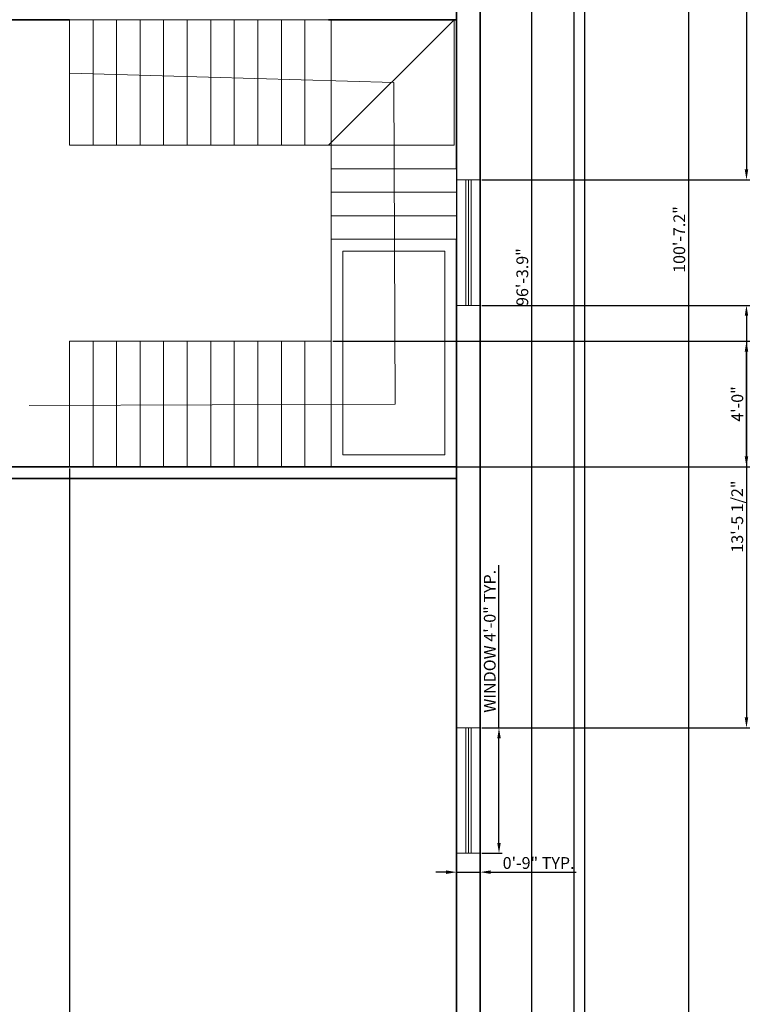
# Model space of a CAD drawing. Units: inches. Extents: x 1239 to 2276906, y 2273 to 321338.
# Tile 14 of 23: x 1754 to 2036, y 2650 to 3026. Entities that reach past the tile are written whole.
import ezdxf

# ---------------------------------------------------------------- set-up
doc = ezdxf.new("R2010")
doc.units = ezdxf.units.IN
for name, color, linetype, lineweight in [('A-ANNO-DIMS', 2, 'Continuous', 18), ('C-PROP', 7, 'Continuous', 25), ('STAIRCASE', 3, 'Continuous', 18), ('wall', 7, 'Continuous', 35), ('WINDOW', 50, 'Continuous', 18)]:
    doc.layers.add(name, color=color, linetype=linetype, lineweight=lineweight)
doc.styles.get("Standard").update_dxf_attribs({"font": 'arial.ttf'})
doc.dimstyles.new('ISO-25', dxfattribs={"dimtxt": 4.5, "dimasz": 4, "dimexe": 1.25, "dimexo": 0.625, "dimtad": 1, "dimdec": 1, "dimlunit": 3, "dimtxsty": 'Standard', "dimcen": 2.5, "dimadec": 0, "dimazin": 0, "dimtfac": 1, "dimtdec": 1, "dimtmove": 0, "dimatfit": 3, "dimfxl": 1, "dimarcsym": 0})

# ---------------------------------------------------------------- blocks, each defined once
blk = doc.blocks.new('*D38')
at = {"layer": 'A-ANNO-DIMS', "color": 0, "lineweight": -2, "transparency": 16777216}
for p, q in [((1971.01, 3545.9), (2011.25, 3545.9)), ((2010, 3541.9), (2010, 2342.75)), ((1971.01, 2338.75), (2011.25, 2338.75))]:
    blk.add_line(p, q, dxfattribs=at)
at = {"layer": 'A-ANNO-DIMS', "color": 0, "transparency": 16777216}
for points in [[(2009.33, 3541.9), (2010.67, 3541.9), (2010, 3545.9)], [(2009.33, 2342.75), (2010.67, 2342.75), (2010, 2338.75)]]:
    blk.add_solid(points, dxfattribs=at)
at = {"layer": 'Defpoints', "color": 0, "transparency": 16777216}
for p in [(1970.38, 3545.9), (1970.38, 2338.75), (2010, 2338.75)]:
    blk.add_point(p, dxfattribs=at)
at = {"layer": 'A-ANNO-DIMS', "color": 0, "transparency": 16777216, "insert": (2007.08, 2942.32), "char_height": 4.5, "attachment_point": 5, "rotation": 90}
blk.add_mtext('100\'-7.2"', dxfattribs=at)
blk = doc.blocks.new('*D40')
at = {"layer": 'A-ANNO-DIMS', "color": 0, "lineweight": -2, "transparency": 16777216}
for p, q in [((1931.01, 3505.9), (1951.25, 3505.9)), ((1950, 3501.9), (1950, 2354)), ((1931.01, 2350), (1951.25, 2350))]:
    blk.add_line(p, q, dxfattribs=at)
at = {"layer": 'A-ANNO-DIMS', "color": 0, "transparency": 16777216}
for points in [[(1949.33, 3501.9), (1950.67, 3501.9), (1950, 3505.9)], [(1949.33, 2354), (1950.67, 2354), (1950, 2350)]]:
    blk.add_solid(points, dxfattribs=at)
at = {"layer": 'Defpoints', "color": 0, "transparency": 16777216}
for p in [(1930.38, 3505.9), (1930.38, 2350), (1950, 2350)]:
    blk.add_point(p, dxfattribs=at)
at = {"layer": 'A-ANNO-DIMS', "color": 0, "transparency": 16777216, "insert": (1947.08, 2927.95), "char_height": 4.5, "attachment_point": 5, "rotation": 90}
blk.add_mtext('96\'-3.9"', dxfattribs=at)
blk = doc.blocks.new('WIN-48')
for p, q in [((0, 48), (9, 48)), ((0, 0), (0, 48)), ((3.5, 0), (3.5, 48)), ((4.5, 0), (4.5, 48)), ((5.5, 0), (5.5, 48)), ((9, 0), (9, 48)), ((0, 0), (9, 0))]:
    blk.add_line(p, q)
blk = doc.blocks.new('*D46')
at = {"layer": 'A-ANNO-DIMS', "color": 0, "lineweight": -2, "transparency": 16777216}
for p, q in [((1937.58, 2755.54), (1937.58, 2817.73)), ((1931.01, 2755.54), (1938.83, 2755.54)), ((1937.58, 2711.54), (1937.58, 2751.54)), ((1931.01, 2707.54), (1938.83, 2707.54))]:
    blk.add_line(p, q, dxfattribs=at)
at = {"layer": 'A-ANNO-DIMS', "color": 0, "transparency": 16777216}
for points in [[(1936.92, 2751.54), (1938.25, 2751.54), (1937.58, 2755.54)], [(1936.92, 2711.54), (1938.25, 2711.54), (1937.58, 2707.54)]]:
    blk.add_solid(points, dxfattribs=at)
at = {"layer": 'Defpoints', "color": 0, "transparency": 16777216}
for p in [(1930.38, 2755.54), (1937.58, 2755.54), (1930.38, 2707.54)]:
    blk.add_point(p, dxfattribs=at)
at = {"layer": 'A-ANNO-DIMS', "color": 0, "transparency": 16777216, "insert": (1934.63, 2788.64), "char_height": 4.5, "attachment_point": 5, "rotation": 90}
blk.add_mtext('WINDOW 4\'-0" TYP.', dxfattribs=at)
blk = doc.blocks.new('*D47')
at = {"layer": 'A-ANNO-DIMS', "color": 0, "lineweight": -2, "transparency": 16777216}
for p, q in [((1921.38, 2706.91), (1921.38, 2699.09)), ((1930.38, 2706.91), (1930.38, 2699.09)), ((1917.38, 2700.34), (1913.38, 2700.34)), ((1921.38, 2700.34), (1930.38, 2700.34)), ((1934.38, 2700.34), (1967.06, 2700.34))]:
    blk.add_line(p, q, dxfattribs=at)
at = {"layer": 'A-ANNO-DIMS', "color": 0, "transparency": 16777216}
for points in [[(1917.38, 2701.01), (1917.38, 2699.67), (1921.38, 2700.34)], [(1934.38, 2701.01), (1934.38, 2699.67), (1930.38, 2700.34)]]:
    blk.add_solid(points, dxfattribs=at)
at = {"layer": 'Defpoints', "color": 0, "transparency": 16777216}
for p in [(1921.38, 2707.54), (1930.38, 2707.54), (1930.38, 2700.34)]:
    blk.add_point(p, dxfattribs=at)
at = {"layer": 'A-ANNO-DIMS', "color": 0, "transparency": 16777216, "insert": (1952.72, 2703.26), "char_height": 4.5, "attachment_point": 5}
blk.add_mtext('0\'-9" TYP.', dxfattribs=at)
blk = doc.blocks.new('*D87')
at = {"layer": 'A-ANNO-DIMS', "color": 0, "lineweight": -2, "transparency": 16777216}
for p, q in [((1666.38, 3250.77), (1666.38, 2275.7)), ((1921.38, 3250.77), (1921.38, 2275.7)), ((1670.38, 2276.95), (1917.38, 2276.95))]:
    blk.add_line(p, q, dxfattribs=at)
at = {"layer": 'A-ANNO-DIMS', "color": 0, "transparency": 16777216}
for points in [[(1670.38, 2277.61), (1670.38, 2276.28), (1666.38, 2276.95)], [(1917.38, 2277.61), (1917.38, 2276.28), (1921.38, 2276.95)]]:
    blk.add_solid(points, dxfattribs=at)
at = {"layer": 'Defpoints', "color": 0, "transparency": 16777216}
for p in [(1666.38, 3251.4), (1921.38, 3251.4), (1921.38, 2276.95)]:
    blk.add_point(p, dxfattribs=at)
at = {"layer": 'A-ANNO-DIMS', "color": 0, "transparency": 16777216, "insert": (1793.88, 2279.87), "char_height": 4.5, "attachment_point": 5}
blk.add_mtext('21\'-3"', dxfattribs=at)
blk = doc.blocks.new('*D98')
at = {"layer": 'A-ANNO-DIMS', "color": 0, "lineweight": -2, "transparency": 16777216}
for p, q in [((1772.76, 3026.4), (1247.33, 3026.4)), ((1248.58, 2859.4), (1248.58, 3022.4)), ((1772.76, 2855.4), (1247.33, 2855.4))]:
    blk.add_line(p, q, dxfattribs=at)
at = {"layer": 'A-ANNO-DIMS', "color": 0, "transparency": 16777216}
for points in [[(1247.92, 3022.4), (1249.25, 3022.4), (1248.58, 3026.4)], [(1247.92, 2859.4), (1249.25, 2859.4), (1248.58, 2855.4)]]:
    blk.add_solid(points, dxfattribs=at)
at = {"layer": 'Defpoints', "color": 0, "transparency": 16777216}
for p in [(1248.58, 3026.4), (1773.38, 3026.4), (1773.38, 2855.4)]:
    blk.add_point(p, dxfattribs=at)
at = {"layer": 'A-ANNO-DIMS', "color": 0, "transparency": 16777216, "insert": (1245.66, 2940.9), "char_height": 4.5, "attachment_point": 5, "rotation": 90}
blk.add_mtext('14\'-3"', dxfattribs=at)
blk = doc.blocks.new('*D99')
at = {"layer": 'A-ANNO-DIMS', "color": 0, "lineweight": -2, "transparency": 16777216}
for p, q in [((1773.38, 2854.77), (1773.38, 2275.7)), ((1921.38, 2854.77), (1921.38, 2275.7)), ((1777.38, 2276.95), (1917.38, 2276.95))]:
    blk.add_line(p, q, dxfattribs=at)
at = {"layer": 'A-ANNO-DIMS', "color": 0, "transparency": 16777216}
for points in [[(1777.38, 2277.61), (1777.38, 2276.28), (1773.38, 2276.95)], [(1917.38, 2277.61), (1917.38, 2276.28), (1921.38, 2276.95)]]:
    blk.add_solid(points, dxfattribs=at)
at = {"layer": 'Defpoints', "color": 0, "transparency": 16777216}
for p in [(1773.38, 2855.4), (1921.38, 2855.4), (1921.38, 2276.95)]:
    blk.add_point(p, dxfattribs=at)
at = {"layer": 'A-ANNO-DIMS', "color": 0, "transparency": 16777216, "insert": (1847.38, 2279.83), "char_height": 4.5, "attachment_point": 5}
blk.add_mtext('12\'-4"', dxfattribs=at)
blk = doc.blocks.new('*D109')
at = {"layer": 'A-ANNO-DIMS', "color": 0, "lineweight": -2, "transparency": 16777216}
for p, q in [((1931.01, 3298.46), (2033.43, 3298.46)), ((2032.18, 3294.46), (2032.18, 2969.13)), ((1931.01, 2965.13), (2033.43, 2965.13))]:
    blk.add_line(p, q, dxfattribs=at)
at = {"layer": 'A-ANNO-DIMS', "color": 0, "transparency": 16777216}
for points in [[(2031.52, 3294.46), (2032.85, 3294.46), (2032.18, 3298.46)], [(2031.52, 2969.13), (2032.85, 2969.13), (2032.18, 2965.13)]]:
    blk.add_solid(points, dxfattribs=at)
at = {"layer": 'Defpoints', "color": 0, "transparency": 16777216}
for p in [(1930.38, 3298.46), (1930.38, 2965.13), (2032.18, 2965.13)]:
    blk.add_point(p, dxfattribs=at)
at = {"layer": 'A-ANNO-DIMS', "color": 0, "transparency": 16777216, "insert": (2029.23, 3131.8), "char_height": 4.5, "attachment_point": 5, "rotation": 90}
blk.add_mtext('27\'-9 1/2"', dxfattribs=at)
blk = doc.blocks.new('*D110')
at = {"layer": 'A-ANNO-DIMS', "color": 0, "lineweight": -2, "transparency": 16777216}
for p, q in [((1931.01, 2917.13), (2033.43, 2917.13)), ((2032.18, 2913.13), (2032.18, 2759.54)), ((1931.01, 2755.54), (2033.43, 2755.54))]:
    blk.add_line(p, q, dxfattribs=at)
at = {"layer": 'A-ANNO-DIMS', "color": 0, "transparency": 16777216}
for points in [[(2031.52, 2913.13), (2032.85, 2913.13), (2032.18, 2917.13)], [(2031.52, 2759.54), (2032.85, 2759.54), (2032.18, 2755.54)]]:
    blk.add_solid(points, dxfattribs=at)
at = {"layer": 'Defpoints', "color": 0, "transparency": 16777216}
for p in [(1930.38, 2917.13), (1930.38, 2755.54), (2032.18, 2755.54)]:
    blk.add_point(p, dxfattribs=at)
at = {"layer": 'A-ANNO-DIMS', "color": 0, "transparency": 16777216, "insert": (2029.23, 2836.34), "char_height": 4.5, "attachment_point": 5, "rotation": 90}
blk.add_mtext('13\'-5 1/2"', dxfattribs=at)
blk = doc.blocks.new('*D115')
at = {"layer": 'A-ANNO-DIMS', "color": 0, "lineweight": -2, "transparency": 16777216}
for p, q in [((1874.01, 2903.4), (2033.43, 2903.4)), ((2032.18, 2859.4), (2032.18, 2899.4)), ((1874.01, 2855.4), (2033.43, 2855.4))]:
    blk.add_line(p, q, dxfattribs=at)
at = {"layer": 'A-ANNO-DIMS', "color": 0, "transparency": 16777216}
for points in [[(2031.52, 2899.4), (2032.85, 2899.4), (2032.18, 2903.4)], [(2031.52, 2859.4), (2032.85, 2859.4), (2032.18, 2855.4)]]:
    blk.add_solid(points, dxfattribs=at)
at = {"layer": 'Defpoints', "color": 0, "transparency": 16777216}
for p in [(1873.38, 2903.4), (2032.18, 2903.4), (1873.38, 2855.4)]:
    blk.add_point(p, dxfattribs=at)
at = {"layer": 'A-ANNO-DIMS', "color": 0, "transparency": 16777216, "insert": (2029.26, 2879.4), "char_height": 4.5, "attachment_point": 5, "rotation": 90}
blk.add_mtext('4\'-0"', dxfattribs=at)

msp = doc.modelspace()

# ---------------------------------------------------------------- linework, layer by layer
at = {"layer": 'C-PROP'}
for points in [[(1970.38, 2345.9), (1970.38, 3545.9), (1310.38, 3545.9), (1310.38, 2345.9), (1644.79, 2345.9)], [(1966.38, 2349.9), (1966.38, 3541.9), (1314.38, 3541.9), (1314.38, 2607.52)]]:
    msp.add_lwpolyline(points, dxfattribs=at)
at = {"layer": 'STAIRCASE'}
for p, q in [((1773.38, 3026.4), (1773.38, 2985.44)), ((1773.38, 3026.4), (1773.38, 2978.4)), ((1782.38, 3026.4), (1773.38, 3026.4)), ((1782.38, 3026.4), (1782.38, 2978.4)), ((1782.38, 3026.4), (1791.38, 3026.4)), ((1791.38, 3026.4), (1791.38, 2978.4)), ((1791.38, 3026.4), (1800.38, 3026.4)), ((1800.38, 3026.4), (1800.38, 2978.4)), ((1800.38, 3026.4), (1809.38, 3026.4)), ((1809.38, 3026.4), (1809.38, 2978.4)), ((1809.38, 3026.4), (1818.38, 3026.4)), ((1818.38, 3026.4), (1818.38, 2978.4)), ((1818.38, 3026.4), (1827.38, 3026.4)), ((1827.38, 3026.4), (1827.38, 2978.4)), ((1827.38, 3026.4), (1836.38, 3026.4)), ((1836.38, 3026.4), (1836.38, 2978.4)), ((1836.38, 3026.4), (1845.38, 3026.4)), ((1845.38, 3026.4), (1845.38, 2978.4)), ((1845.38, 3026.4), (1854.38, 3026.4)), ((1854.38, 3026.4), (1854.38, 2978.4)), ((1854.38, 3026.4), (1863.38, 3026.4)), ((1863.38, 3026.4), (1872.38, 3026.4)), ((1863.38, 3026.4), (1863.38, 2978.4)), ((1920.38, 3026.4), (1872.38, 3026.4)), ((1920.38, 3026.4), (1872.38, 2978.4)), ((1873.38, 2978.4), (1873.38, 3026.4)), ((1920.38, 2978.4), (1920.38, 3026.4)), ((1773.38, 3005.92), (1773.38, 3005.92)), ((1773.38, 3005.92), (1897.38, 3002.4)), ((1897.38, 3002.4), (1897.83, 2879.4)), ((1773.38, 2978.4), (1782.38, 2978.4)), ((1782.38, 2978.4), (1791.38, 2978.4)), ((1791.38, 2978.4), (1800.38, 2978.4)), ((1800.38, 2978.4), (1809.38, 2978.4)), ((1809.38, 2978.4), (1818.38, 2978.4)), ((1818.38, 2978.4), (1827.38, 2978.4)), ((1827.38, 2978.4), (1836.38, 2978.4)), ((1836.38, 2978.4), (1845.38, 2978.4)), ((1845.38, 2978.4), (1854.38, 2978.4)), ((1854.38, 2978.4), (1863.38, 2978.4)), ((1863.38, 2978.4), (1872.38, 2978.4)), ((1872.38, 2978.4), (1920.38, 2978.4)), ((1872.38, 2978.4), (1920.38, 2978.4)), ((1873.38, 2942.4), (1873.38, 2978.4)), ((1873.38, 2969.4), (1921.38, 2969.4)), ((1921.38, 2969.4), (1921.38, 2960.4)), ((1873.38, 2960.4), (1921.38, 2960.4)), ((1921.38, 2960.4), (1921.38, 2951.4)), ((1873.38, 2951.4), (1921.38, 2951.4)), ((1921.38, 2951.4), (1921.38, 2942.4)), ((1873.38, 2942.4), (1921.38, 2942.4)), ((1773.38, 2903.4), (1773.38, 2855.4)), ((1782.38, 2903.4), (1773.38, 2903.4)), ((1773.38, 2903.4), (1773.38, 2862.44)), ((1782.38, 2903.4), (1782.38, 2855.4)), ((1782.38, 2903.4), (1791.38, 2903.4)), ((1791.38, 2903.4), (1791.38, 2855.4)), ((1791.38, 2903.4), (1800.38, 2903.4)), ((1800.38, 2903.4), (1800.38, 2855.4)), ((1800.38, 2903.4), (1809.38, 2903.4)), ((1809.38, 2903.4), (1809.38, 2855.4)), ((1809.38, 2903.4), (1818.38, 2903.4)), ((1818.38, 2903.4), (1818.38, 2855.4)), ((1818.38, 2903.4), (1827.38, 2903.4)), ((1827.38, 2903.4), (1827.38, 2855.4)), ((1827.38, 2903.4), (1836.38, 2903.4)), ((1836.38, 2903.4), (1836.38, 2855.4)), ((1836.38, 2903.4), (1845.38, 2903.4)), ((1845.38, 2903.4), (1845.38, 2855.4)), ((1845.38, 2903.4), (1854.38, 2903.4)), ((1854.38, 2903.4), (1854.38, 2855.4)), ((1854.38, 2903.4), (1863.38, 2903.4)), ((1863.38, 2903.4), (1863.38, 2855.4)), ((1863.38, 2903.4), (1873.38, 2903.4)), ((1873.38, 2855.4), (1873.38, 2903.4)), ((1897.83, 2879.4), (1758.03, 2878.88)), ((1773.38, 2855.4), (1782.38, 2855.4)), ((1782.38, 2855.4), (1791.38, 2855.4)), ((1791.38, 2855.4), (1800.38, 2855.4)), ((1800.38, 2855.4), (1809.38, 2855.4)), ((1809.38, 2855.4), (1818.38, 2855.4)), ((1818.38, 2855.4), (1827.38, 2855.4)), ((1827.38, 2855.4), (1836.38, 2855.4)), ((1836.38, 2855.4), (1845.38, 2855.4)), ((1845.38, 2855.4), (1854.38, 2855.4)), ((1854.38, 2855.4), (1863.38, 2855.4))]:
    msp.add_line(p, q, dxfattribs=at)
for points in [[(1873.38, 2942.4), (1921.38, 2942.4), (1921.38, 2855.4), (1873.38, 2855.4)], [(1877.88, 2937.9), (1916.88, 2937.9), (1916.88, 2859.9), (1877.88, 2859.9)]]:
    msp.add_lwpolyline(points, close=True, dxfattribs=at)
at = {"layer": 'wall'}
for p, q in [((1930.38, 2385.9), (1930.38, 3505.9)), ((1921.38, 2969.4), (1921.38, 3407.4)), ((1773.38, 3026.4), (1620.71, 3026.4)), ((1921.38, 3026.4), (1872.38, 3026.4)), ((1921.38, 2394.9), (1921.38, 2942.4)), ((1773.38, 2855.4), (1555.88, 2855.4)), ((1921.38, 2855.4), (1666.38, 2855.4)), ((1921.38, 2850.9), (1666.38, 2850.9))]:
    msp.add_line(p, q, dxfattribs=at)

# ---------------------------------------------------------------- block references
at = {"layer": 'WINDOW'}
for p in [(1921.38, 2917.13), (1921.38, 2707.54)]:
    msp.add_blockref('WIN-48', p, dxfattribs=at)

# ---------------------------------------------------------------- dimensions: what is measured, and where the dimension line sits
at = {"layer": 'A-ANNO-DIMS'}
for base, p1, p2, override, picture, middle in [((2010, 2338.7461), (1970.3833, 3545.8972), (1970.3833, 2338.7461), {"dimclrd": 0, "dimclre": 0, "dimclrt": 0}, '*D38', (2007.0774, 2942.3216)), ((1950, 2350), (1930.38, 3505.9), (1930.38, 2350), {"dimclrd": 0, "dimclre": 0, "dimclrt": 0}, '*D40', (1947.08, 2927.95)), ((2032.18, 2965.13), (1930.38, 3298.46), (1930.38, 2965.13), {"dimdec": 1, "dimlfac": 1, "dimrnd": 0, "dimzin": 1, "dimdsep": 46, "dimlunit": 4, "dimfrac": 2}, '*D109', (2029.23, 3131.8)), ((1248.58, 3026.4), (1773.38, 2855.4), (1773.38, 3026.4), {"dimdec": 1, "dimlfac": 1, "dimrnd": 0, "dimzin": 1, "dimdsep": 46, "dimlunit": 4, "dimfrac": 2}, '*D98', (1245.66, 2940.9)), ((2032.18, 2755.54), (1930.38, 2917.13), (1930.38, 2755.54), {"dimdec": 1, "dimlfac": 1, "dimrnd": 0, "dimzin": 1, "dimdsep": 46, "dimlunit": 4, "dimfrac": 2}, '*D110', (2029.23, 2836.34)), ((2032.18, 2903.4), (1873.38, 2855.4), (1873.38, 2903.4), {"dimdec": 1, "dimlfac": 1, "dimrnd": 0, "dimzin": 1, "dimdsep": 46, "dimlunit": 4, "dimfrac": 2}, '*D115', (2029.26, 2879.4))]:
    dim = msp.add_linear_dim(base=base, p1=p1, p2=p2, angle=90, dimstyle='ISO-25', override=override, dxfattribs=at)
    dim.commit()
    dim.dimension.update_dxf_attribs({"geometry": picture, "text_midpoint": middle})
for p1, p2, picture, middle in [((1666.38, 3251.4), (1921.38, 3251.4), '*D87', (1793.88, 2279.87)), ((1773.38, 2855.4), (1921.38, 2855.4), '*D99', (1847.38, 2279.83))]:
    dim = msp.add_linear_dim(base=(1921.38, 2276.95), p1=p1, p2=p2, dimstyle='ISO-25', override={"dimdec": 1, "dimlfac": 1, "dimrnd": 0, "dimzin": 1, "dimdsep": 46, "dimlunit": 4, "dimfrac": 2}, dxfattribs=at)
    dim.commit()
    dim.dimension.update_dxf_attribs({"geometry": picture, "text_midpoint": middle})
dim = msp.add_linear_dim(base=(1937.58, 2755.54), p1=(1930.38, 2707.54), p2=(1930.38, 2755.54), angle=90, text='WINDOW <> TYP.', dimstyle='ISO-25', override={"dimdec": 1, "dimlfac": 1, "dimrnd": 0, "dimzin": 1, "dimdsep": 46, "dimlunit": 4, "dimfrac": 2}, dxfattribs=at)
dim.commit()
dim.dimension.update_dxf_attribs({"geometry": '*D46', "text_midpoint": (1934.63, 2788.64)})
dim = msp.add_linear_dim(base=(1930.38, 2700.34), p1=(1921.38, 2707.54), p2=(1930.38, 2707.54), text='<> TYP.', dimstyle='ISO-25', override={"dimdec": 1, "dimlfac": 1, "dimrnd": 0, "dimzin": 1, "dimdsep": 46, "dimlunit": 4, "dimfrac": 2}, dxfattribs=at)
dim.commit()
dim.dimension.update_dxf_attribs({"geometry": '*D47', "text_midpoint": (1952.72, 2703.26)})

doc.saveas('drawing.dxf')
